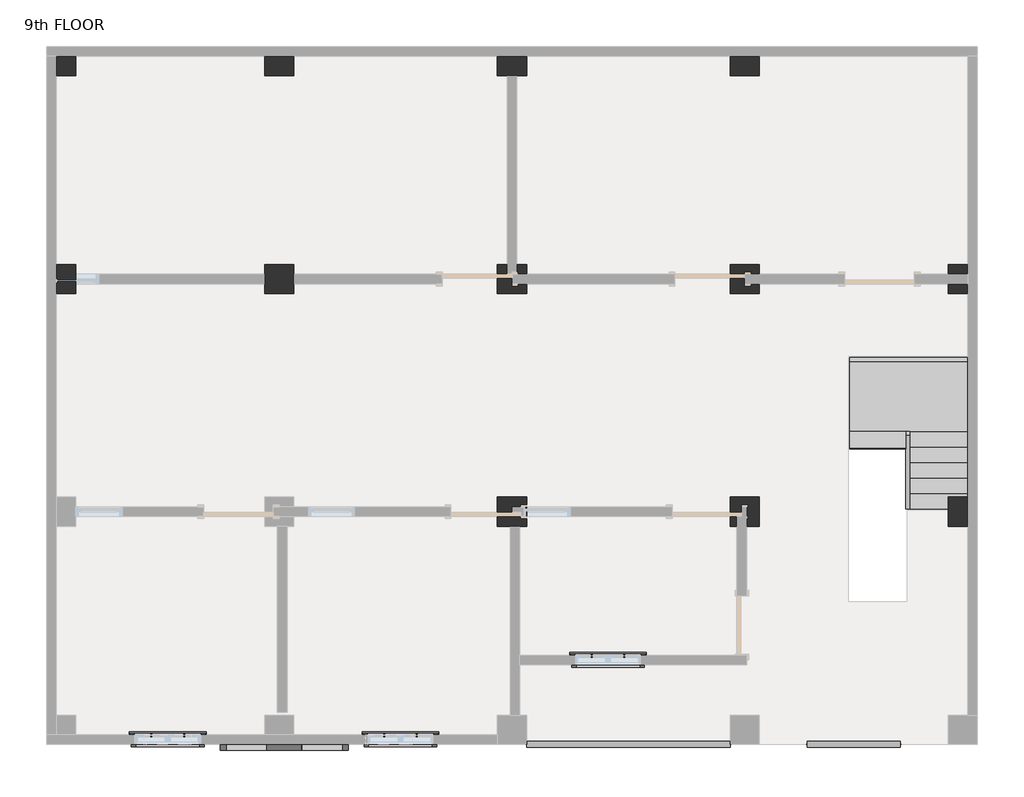
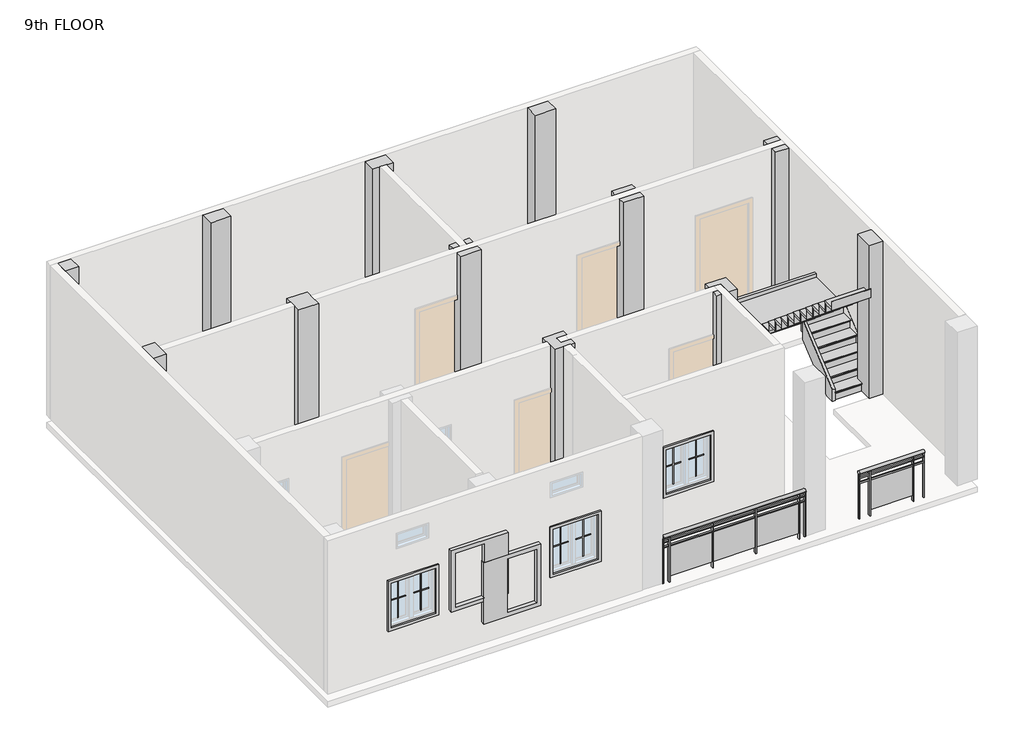
# One storey, part 2 of 2: 12 columns, 12 proxies, 4 members, 2 railings, 1 damper, 1 stair flight.
"""IFC4 building model written with IfcOpenShell, lengths in millimetres."""

from ifc_helpers import new_model, si_unit, point, frame, origin, place, context, project, spatial, polyline, ellipse_curve, trimmed, outline, extrude, faceted_brep, transform, mapped, element, save
from ifc_brep_helpers import plane_surface, extruded_surface, advanced_brep
from components import muntin_pattern_2x2_muntin_pattern_2x2_b3fe6957, muntin_pattern_2x2_muntin_pattern_2x2_3e0ecaf2, trim_window_exterior_flat_with_sill_41619996, trim_window_interior_flat_picture_frame_51c85655, duct_accessories_4_duct_accessories_1_42753040, stair_flight_cacad448

model = new_model("IFC4")

# Units and contexts
model_context = context("Model", 3, world=origin())
ifc_project = project(units=[si_unit("LENGTHUNIT", "METRE", prefix="MILLI")], contexts=[model_context])

# Site, building, storey
site = spatial("IfcSite", under=ifc_project)
building = spatial("IfcBuilding", under=site)
storey = spatial("IfcBuildingStorey", under=building, Name="9th FLOOR", Elevation=27279.6)

# Proxies
placement = place(None, origin())
muntin_pattern_2x2_muntin_pattern_2x2_shape = muntin_pattern_2x2_muntin_pattern_2x2_b3fe6957(model_context)
element("IfcBuildingElementProxy", 1, Name="Muntin Pattern_2x2 : Muntin Pattern_2x2", ObjectType="Muntin Pattern_2x2 : Muntin Pattern_2x2", at=placement, inside=storey, context=model_context, shape_type="MappedRepresentation", body=[
    mapped(muntin_pattern_2x2_muntin_pattern_2x2_shape, transform((-14441.409625, -253.8184478, 28263.85), x_axis=(1.0, 0.0, 0.0), y_axis=(0.0, 1.0, 0.0), z_axis=(0.0, 0.0, 1.0))),
])
element("IfcBuildingElementProxy", 2, Name="Muntin Pattern_2x2 : Muntin Pattern_2x2", ObjectType="Muntin Pattern_2x2 : Muntin Pattern_2x2", at=placement, inside=storey, context=model_context, shape_type="MappedRepresentation", body=[
    mapped(muntin_pattern_2x2_muntin_pattern_2x2_shape, transform((-11393.409625, -253.8184478, 28263.85), x_axis=(1.0, 0.0, 0.0), y_axis=(0.0, 1.0, 0.0), z_axis=(0.0, 0.0, 1.0))),
])
element("IfcBuildingElementProxy", 3, Name="Muntin Pattern_2x2 : Muntin Pattern_2x2", ObjectType="Muntin Pattern_2x2 : Muntin Pattern_2x2", at=placement, inside=storey, context=model_context, shape_type="MappedRepresentation", body=[
    mapped(muntin_pattern_2x2_muntin_pattern_2x2_shape, transform((-8675.609625, 787.5815522, 28263.85), x_axis=(1.0, 0.0, 0.0), y_axis=(0.0, 1.0, 0.0), z_axis=(0.0, 0.0, 1.0))),
])
muntin_pattern_2x2_muntin_pattern_2x2_2_shape = muntin_pattern_2x2_muntin_pattern_2x2_3e0ecaf2(model_context)
element("IfcBuildingElementProxy", 4, Name="Muntin Pattern_2x2 : Muntin Pattern_2x2", ObjectType="Muntin Pattern_2x2 : Muntin Pattern_2x2", at=placement, inside=storey, context=model_context, shape_type="MappedRepresentation", body=[
    mapped(muntin_pattern_2x2_muntin_pattern_2x2_2_shape, transform((-14012.784625, -253.8184478, 28263.85), x_axis=(-1.0, 0.0, 0.0), y_axis=(0.0, -1.0, 0.0), z_axis=(0.0, 0.0, 1.0))),
])
element("IfcBuildingElementProxy", 5, Name="Muntin Pattern_2x2 : Muntin Pattern_2x2", ObjectType="Muntin Pattern_2x2 : Muntin Pattern_2x2", at=placement, inside=storey, context=model_context, shape_type="MappedRepresentation", body=[
    mapped(muntin_pattern_2x2_muntin_pattern_2x2_2_shape, transform((-10964.784625, -253.8184478, 28263.85), x_axis=(-1.0, 0.0, 0.0), y_axis=(0.0, -1.0, 0.0), z_axis=(0.0, 0.0, 1.0))),
])
element("IfcBuildingElementProxy", 6, Name="Muntin Pattern_2x2 : Muntin Pattern_2x2", ObjectType="Muntin Pattern_2x2 : Muntin Pattern_2x2", at=placement, inside=storey, context=model_context, shape_type="MappedRepresentation", body=[
    mapped(muntin_pattern_2x2_muntin_pattern_2x2_2_shape, transform((-8246.984625, 787.5815522, 28263.85), x_axis=(-1.0, 0.0, 0.0), y_axis=(0.0, -1.0, 0.0), z_axis=(0.0, 0.0, 1.0))),
])
trim_window_exterior_flat_with_sill_shape = trim_window_exterior_flat_with_sill_41619996(model_context)
element("IfcBuildingElementProxy", 7, Name="Trim-Window-Exterior-Flat : with Sill", ObjectType="Trim-Window-Exterior-Flat : with Sill", at=placement, inside=storey, context=model_context, shape_type="MappedRepresentation", body=[
    mapped(trim_window_exterior_flat_with_sill_shape, transform((-14227.097125, -244.2934478, 29108.4), x_axis=(-1.0, 0.0, 0.0), y_axis=(0.0, 0.0, 1.0), z_axis=(0.0, 1.0, 0.0))),
])
element("IfcBuildingElementProxy", 8, Name="Trim-Window-Exterior-Flat : with Sill", ObjectType="Trim-Window-Exterior-Flat : with Sill", at=placement, inside=storey, context=model_context, shape_type="MappedRepresentation", body=[
    mapped(trim_window_exterior_flat_with_sill_shape, transform((-11179.097125, -244.2934478, 29108.4), x_axis=(-1.0, 0.0, 0.0), y_axis=(0.0, 0.0, 1.0), z_axis=(0.0, 1.0, 0.0))),
])
element("IfcBuildingElementProxy", 9, Name="Trim-Window-Exterior-Flat : with Sill", ObjectType="Trim-Window-Exterior-Flat : with Sill", at=placement, inside=storey, context=model_context, shape_type="MappedRepresentation", body=[
    mapped(trim_window_exterior_flat_with_sill_shape, transform((-8461.297125, 797.1065522, 29108.4), x_axis=(-1.0, 0.0, 0.0), y_axis=(0.0, 0.0, 1.0), z_axis=(0.0, 1.0, 0.0))),
])
trim_window_interior_flat_picture_frame_shape = trim_window_interior_flat_picture_frame_51c85655(model_context)
element("IfcBuildingElementProxy", 10, Name="Trim-Window-Interior-Flat : Picture Frame", ObjectType="Trim-Window-Interior-Flat : Picture Frame", at=placement, inside=storey, context=model_context, shape_type="MappedRepresentation", body=[
    mapped(trim_window_interior_flat_picture_frame_shape, transform((-14227.097125, -371.2934478, 29108.4), x_axis=(1.0, 0.0, 0.0), y_axis=(0.0, 0.0, 1.0), z_axis=(0.0, -1.0, 0.0))),
])
element("IfcBuildingElementProxy", 11, Name="Trim-Window-Interior-Flat : Picture Frame", ObjectType="Trim-Window-Interior-Flat : Picture Frame", at=placement, inside=storey, context=model_context, shape_type="MappedRepresentation", body=[
    mapped(trim_window_interior_flat_picture_frame_shape, transform((-11179.097125, -371.2934478, 29108.4), x_axis=(1.0, 0.0, 0.0), y_axis=(0.0, 0.0, 1.0), z_axis=(0.0, -1.0, 0.0))),
])
element("IfcBuildingElementProxy", 12, Name="Trim-Window-Interior-Flat : Picture Frame", ObjectType="Trim-Window-Interior-Flat : Picture Frame", at=placement, inside=storey, context=model_context, shape_type="MappedRepresentation", body=[
    mapped(trim_window_interior_flat_picture_frame_shape, transform((-8461.297125, 670.1065522, 29108.4), x_axis=(1.0, 0.0, 0.0), y_axis=(0.0, 0.0, 1.0), z_axis=(0.0, -1.0, 0.0))),
])

# Columns
element("IfcColumn", 13, ObjectType="column family : column family", at=placement, inside=storey, context=model_context, shape_type="SweptSolid", body=[
    extrude(outline(polyline([(-15433.597125, 8645.7065522), (-15433.597125, 8391.7065522), (-15687.597125, 8391.7065522), (-15687.597125, 8645.7065522), (-15433.597125, 8645.7065522)])), frame((0.0, 0.0, 27284.6), z_axis=(0.0, 0.0, 1.0), x_axis=(1.0, 0.0, 0.0)), (0.0, 0.0, 1.0), 3038.0),
])
element("IfcColumn", 14, ObjectType="column family : column family", at=placement, inside=storey, context=model_context, shape_type="SweptSolid", body=[
    extrude(outline(polyline([(-12576.097125, 5915.2065522), (-12576.097125, 5534.2065522), (-12957.097125, 5534.2065522), (-12957.097125, 5915.2065522), (-12576.097125, 5915.2065522)])), frame((0.0, 0.0, 27284.6), z_axis=(0.0, 0.0, 1.0), x_axis=(1.0, 0.0, 0.0)), (0.0, 0.0, 1.0), 3038.0),
])
element("IfcColumn", 15, ObjectType="column family : column family", at=placement, inside=storey, context=model_context, shape_type="Brep", body=[
    faceted_brep([(-9655.097125, 5915.2065522, 27284.6), (-9528.097125, 5915.2065522, 27284.6), (-9528.097125, 5788.2065522, 27284.6), (-9655.097125, 5788.2065522, 27284.6), (-9528.097125, 5915.2065522, 30322.6), (-9655.097125, 5915.2065522, 30322.6), (-9655.097125, 5788.2065522, 30322.6), (-9528.097125, 5788.2065522, 30322.6)], [[[0, 1, 2, 3]], [[4, 5, 6, 7]], [[0, 3, 6, 5]], [[4, 1, 0, 5]], [[3, 2, 7, 6]], [[1, 4, 7, 2]]]),
    faceted_brep([(-9528.097125, 5534.2065522, 30322.6), (-9528.097125, 5534.2065522, 27284.6), (-9528.097125, 5661.2065522, 27284.6), (-9528.097125, 5661.2065522, 30322.6), (-9909.097125, 5534.2065522, 27284.6), (-9909.097125, 5534.2065522, 30322.6), (-9909.097125, 5915.2065522, 27284.6), (-9909.097125, 5661.2065522, 30322.6), (-9909.097125, 5661.2065522, 29413.2), (-9909.097125, 5788.2065522, 29413.2), (-9909.097125, 5788.2065522, 30322.6), (-9909.097125, 5915.2065522, 30322.6), (-9782.097125, 5915.2065522, 30322.6), (-9782.097125, 5915.2065522, 27284.6), (-9782.097125, 5788.2065522, 27284.6), (-9782.097125, 5788.2065522, 30322.6), (-9782.097125, 5788.2065522, 29413.2), (-9718.597125, 5788.2065522, 27284.6), (-9718.597125, 5788.2065522, 29413.2), (-9718.597125, 5661.2065522, 27284.6), (-9718.597125, 5661.2065522, 29413.2)], [[[0, 1, 2, 3]], [[4, 1, 0, 5]], [[6, 4, 5, 7, 8, 9, 10, 11]], [[6, 11, 12, 13]], [[14, 13, 12, 15, 16]], [[17, 14, 16, 18]], [[19, 20, 8, 7, 3, 2]], [[1, 4, 6, 13, 14, 17, 19, 2]], [[5, 0, 3, 7]], [[12, 11, 10, 15]], [[9, 16, 15, 10]], [[18, 20, 19, 17]], [[20, 18, 16, 9, 8]]]),
])
element("IfcColumn", 16, ObjectType="column family : column family", at=placement, inside=storey, context=model_context, shape_type="Brep", body=[
    faceted_brep([(-6480.097125, 5534.2065522, 27284.6), (-6861.097125, 5534.2065522, 27284.6), (-6861.097125, 5915.2065522, 27284.6), (-6480.097125, 5915.2065522, 27284.6), (-6480.097125, 5788.2065522, 27284.6), (-6670.597125, 5788.2065522, 27284.6), (-6670.597125, 5661.2065522, 27284.6), (-6480.097125, 5661.2065522, 27284.6), (-6480.097125, 5534.2065522, 30322.6), (-6480.097125, 5661.2065522, 30322.6), (-6861.097125, 5534.2065522, 30322.6), (-6861.097125, 5661.2065522, 30322.6), (-6861.097125, 5661.2065522, 29413.2), (-6861.097125, 5788.2065522, 29413.2), (-6861.097125, 5788.2065522, 30322.6), (-6861.097125, 5915.2065522, 30322.6), (-6480.097125, 5915.2065522, 30322.6), (-6670.597125, 5661.2065522, 29413.2), (-6670.597125, 5788.2065522, 29413.2), (-6480.097125, 5788.2065522, 30322.6)], [[[0, 1, 2, 3, 4, 5, 6, 7]], [[8, 0, 7, 9]], [[1, 0, 8, 10]], [[2, 1, 10, 11, 12, 13, 14, 15]], [[3, 2, 15, 16]], [[10, 8, 9, 11]], [[6, 17, 12, 11, 9, 7]], [[13, 18, 5, 4, 19, 14]], [[3, 16, 19, 4]], [[16, 15, 14, 19]], [[18, 17, 6, 5]], [[17, 18, 13, 12]]]),
])
element("IfcColumn", 17, ObjectType="column family : column family", at=placement, inside=storey, context=model_context, shape_type="Brep", body=[
    faceted_brep([(-6480.097125, 2867.2065522, 27284.6), (-6480.097125, 2486.2065522, 27284.6), (-6645.197125, 2486.2065522, 27284.6), (-6645.197125, 2740.2065522, 27284.6), (-6708.697125, 2740.2065522, 27284.6), (-6708.697125, 2613.2065522, 27284.6), (-6772.197125, 2613.2065522, 27284.6), (-6772.197125, 2486.2065522, 27284.6), (-6861.097125, 2486.2065522, 27284.6), (-6861.097125, 2867.2065522, 27284.6), (-6480.097125, 2867.2065522, 30322.6), (-6480.097125, 2486.2065522, 30322.6), (-6861.097125, 2486.2065522, 30322.6), (-6772.197125, 2486.2065522, 30322.6), (-6861.097125, 2613.2065522, 30322.6), (-6861.097125, 2613.2065522, 29413.2), (-6861.097125, 2740.2065522, 29413.2), (-6861.097125, 2740.2065522, 30322.6), (-6861.097125, 2867.2065522, 30322.6), (-6772.197125, 2740.2065522, 30322.6), (-6645.197125, 2740.2065522, 30322.6), (-6645.197125, 2486.2065522, 30322.6), (-6772.197125, 2613.2065522, 30322.6), (-6772.197125, 2613.2065522, 29413.2), (-6772.197125, 2740.2065522, 29413.2), (-6708.697125, 2613.2065522, 29413.2), (-6708.697125, 2740.2065522, 29413.2)], [[[0, 1, 2, 3, 4, 5, 6, 7, 8, 9]], [[1, 0, 10, 11]], [[12, 8, 7, 13]], [[9, 8, 12, 14, 15, 16, 17, 18]], [[0, 9, 18, 10]], [[11, 10, 18, 17, 19, 20, 21]], [[15, 14, 22, 23]], [[17, 16, 24, 19]], [[20, 3, 2, 21]], [[6, 23, 22, 13, 7]], [[14, 12, 13, 22]], [[1, 11, 21, 2]], [[15, 23, 24, 16]], [[25, 23, 6, 5]], [[23, 25, 26, 24]], [[26, 25, 5, 4]], [[24, 26, 4, 3, 20, 19]]]),
])
element("IfcColumn", 18, ObjectType="column family : column family", at=placement, inside=storey, context=model_context, shape_type="Brep", body=[
    faceted_brep([(-9528.097125, 2486.2065522, 27284.6), (-9909.097125, 2486.2065522, 27284.6), (-9909.097125, 2867.2065522, 27284.6), (-9528.097125, 2867.2065522, 27284.6), (-9528.097125, 2740.2065522, 27284.6), (-9566.197125, 2740.2065522, 27284.6), (-9718.597125, 2740.2065522, 27284.6), (-9718.597125, 2613.2065522, 27284.6), (-9566.197125, 2613.2065522, 27284.6), (-9528.097125, 2613.2065522, 27284.6), (-9528.097125, 2486.2065522, 30322.6), (-9528.097125, 2613.2065522, 27584.4), (-9528.097125, 2740.2065522, 27584.4), (-9528.097125, 2867.2065522, 30322.6), (-9528.097125, 2740.2065522, 30322.6), (-9528.097125, 2740.2065522, 29413.2), (-9528.097125, 2613.2065522, 29413.2), (-9528.097125, 2613.2065522, 30322.6), (-9909.097125, 2486.2065522, 30322.6), (-9909.097125, 2867.2065522, 30322.6), (-9566.197125, 2613.2065522, 30322.6), (-9718.597125, 2613.2065522, 30322.6), (-9718.597125, 2740.2065522, 30322.6), (-9566.197125, 2740.2065522, 30322.6), (-9566.197125, 2613.2065522, 29413.2), (-9566.197125, 2613.2065522, 27584.4), (-9566.197125, 2740.2065522, 27584.4), (-9566.197125, 2740.2065522, 29413.2)], [[[0, 1, 2, 3, 4, 5, 6, 7, 8, 9]], [[10, 0, 9, 11, 12, 4, 3, 13, 14, 15, 16, 17]], [[1, 0, 10, 18]], [[2, 1, 18, 19]], [[3, 2, 19, 13]], [[18, 10, 17, 20, 21, 22, 23, 14, 13, 19]], [[11, 9, 8, 7, 21, 20, 17, 16, 24, 25]], [[4, 12, 26, 27, 15, 14, 23, 22, 6, 5]], [[21, 7, 6, 22]], [[25, 24, 27, 26]], [[25, 26, 12, 11]], [[27, 24, 16, 15]]]),
])
element("IfcColumn", 19, ObjectType="column family : column family", at=placement, inside=storey, context=model_context, shape_type="SweptSolid", body=[
    extrude(outline(polyline([(-12576.097125, 8391.7065522), (-12957.097125, 8391.7065522), (-12957.097125, 8645.7065522), (-12576.097125, 8645.7065522), (-12576.097125, 8391.7065522)])), frame((0.0, 0.0, 27284.6), z_axis=(0.0, 0.0, 1.0), x_axis=(1.0, 0.0, 0.0)), (0.0, 0.0, 1.0), 3038.0),
])
element("IfcColumn", 20, ObjectType="column family : column family", at=placement, inside=storey, context=model_context, shape_type="SweptSolid", body=[
    extrude(outline(polyline([(-9528.097125, 8391.7065522), (-9909.097125, 8391.7065522), (-9909.097125, 8645.7065522), (-9528.097125, 8645.7065522), (-9528.097125, 8391.7065522)])), frame((0.0, 0.0, 27284.6), z_axis=(0.0, 0.0, 1.0), x_axis=(1.0, 0.0, 0.0)), (0.0, 0.0, 1.0), 3038.0),
])
element("IfcColumn", 21, ObjectType="column family : column family", at=placement, inside=storey, context=model_context, shape_type="SweptSolid", body=[
    extrude(outline(polyline([(-6480.097125, 8391.7065522), (-6861.097125, 8391.7065522), (-6861.097125, 8645.7065522), (-6480.097125, 8645.7065522), (-6480.097125, 8391.7065522)])), frame((0.0, 0.0, 27284.6), z_axis=(0.0, 0.0, 1.0), x_axis=(1.0, 0.0, 0.0)), (0.0, 0.0, 1.0), 3038.0),
])
element("IfcColumn", 22, ObjectType="column family : column family", at=placement, inside=storey, context=model_context, shape_type="SweptSolid", body=[
    extrude(outline(polyline([(-4003.597125, 5915.2065522), (-3749.597125, 5915.2065522), (-3749.597125, 5788.2065522), (-4003.597125, 5788.2065522), (-4003.597125, 5915.2065522)])), frame((0.0, 0.0, 27284.6), z_axis=(0.0, 0.0, 1.0), x_axis=(1.0, 0.0, 0.0)), (0.0, 0.0, 1.0), 3038.0),
    extrude(outline(polyline([(-3749.597125, 5534.2065522), (-4003.597125, 5534.2065522), (-4003.597125, 5661.2065522), (-3749.597125, 5661.2065522), (-3749.597125, 5534.2065522)])), frame((0.0, 0.0, 27284.6), z_axis=(0.0, 0.0, 1.0), x_axis=(1.0, 0.0, 0.0)), (0.0, 0.0, 1.0), 3038.0),
])
element("IfcColumn", 23, ObjectType="column family : column family", at=placement, inside=storey, context=model_context, shape_type="SweptSolid", body=[
    extrude(outline(polyline([(-4003.597125, 2486.2065522), (-4003.597125, 2867.2065522), (-3749.597125, 2867.2065522), (-3749.597125, 2486.2065522), (-4003.597125, 2486.2065522)])), frame((0.0, 0.0, 27284.6), z_axis=(0.0, 0.0, 1.0), x_axis=(1.0, 0.0, 0.0)), (0.0, 0.0, 1.0), 3038.0),
])
element("IfcColumn", 24, ObjectType="column family : column family", at=placement, inside=storey, context=model_context, shape_type="SweptSolid", body=[
    extrude(outline(polyline([(-15433.597125, 5915.2065522), (-15433.597125, 5534.2065522), (-15687.597125, 5534.2065522), (-15687.597125, 5915.2065522), (-15433.597125, 5915.2065522)])), frame((0.0, 0.0, 27284.6), z_axis=(0.0, 0.0, 1.0), x_axis=(1.0, 0.0, 0.0)), (0.0, 0.0, 1.0), 3038.0),
])

# Damper
duct_accessories_4_duct_accessories_1_shape = duct_accessories_4_duct_accessories_1_42753040(model_context)
element("IfcDamper", 25, ObjectType="Duct Accessories 4 : Duct Accessories 1", at=placement, inside=storey, context=model_context, shape_type="MappedRepresentation", body=[
    mapped(duct_accessories_4_duct_accessories_1_shape, transform((0.0, 0.0, 0.0), x_axis=(1.0, 0.0, 0.0), y_axis=(0.0, 1.0, 0.0), z_axis=(0.0, 0.0, 1.0))),
])

# Members
element("IfcMember", 26, ObjectType="Stringer - 2\" Width", at=placement, inside=storey, context=model_context, shape_type="SweptSolid", body=[
    extrude(outline(polyline([(2714.6319226, 27279.6), (2714.6319226, 27516.4438745), (3679.8319226, 28320.7772078), (3679.8319226, 27924.0165243), (2906.5320935, 27279.6), (2714.6319226, 27279.6)])), frame((-4563.0136682, 0.0, 0.0), z_axis=(1.0, 0.0, 0.0), x_axis=(0.0, 1.0, 0.0)), (0.0, 0.0, 1.0), 50.8),
])
element("IfcMember", 27, ObjectType="Stringer - 2\" Width", at=placement, inside=storey, context=model_context, shape_type="SweptSolid", body=[
    extrude(outline(polyline([(-4512.2136682, 3730.6319226), (-4512.2136682, 3679.8319226), (-4563.0136682, 3679.8319226), (-4563.0136682, 3730.6319226), (-4512.2136682, 3730.6319226)])), frame((0.0, 0.0, 28067.0), z_axis=(0.0, 0.0, 1.0), x_axis=(1.0, 0.0, 0.0)), (0.0, 0.0, 1.0), 304.8),
])
element("IfcMember", 28, ObjectType="Stringer - 2\" Width", at=placement, inside=storey, context=model_context, shape_type="SweptSolid", body=[
    extrude(outline(polyline([(2714.6319226, 27279.6), (2714.6319226, 27516.4438745), (3741.0592732, 28371.8), (4217.1720935, 28371.8), (2906.5320935, 27279.6), (2714.6319226, 27279.6)])), frame((-3749.597125, 0.0, 0.0), z_axis=(1.0, 0.0, 0.0), x_axis=(0.0, 1.0, 0.0)), (0.0, 0.0, 1.0), 50.8),
])
element("IfcMember", 29, ObjectType="Stringer - 2\" Width", at=placement, inside=storey, context=model_context, shape_type="SweptSolid", body=[
    extrude(outline(polyline([(-3698.797125, 4695.8319226), (-3698.797125, 4645.0319226), (-5295.0246464, 4645.0319226), (-5295.0246464, 4695.8319226), (-3698.797125, 4695.8319226)])), frame((0.0, 0.0, 28067.0), z_axis=(0.0, 0.0, 1.0), x_axis=(1.0, 0.0, 0.0)), (0.0, 0.0, 1.0), 304.8),
])

# Railings
element("IfcRailing", 30, ObjectType="Glass Panel - Bottom Fill", at=placement, inside=storey, context=model_context, shape_type="SolidModel", body=[
    advanced_brep(
    [(-9528.097125, -333.1934478, 28194.0), (-9528.097125, -409.3934478, 28194.0), (-6861.097125, -333.1934478, 28194.0), (-6861.097125, -409.3934478, 28194.0)],
    [
        (0, 1, ellipse_curve(frame((-9528.097125, -371.2934478, 28194.0), z_axis=(-1.0, 0.0, 0.0), x_axis=(0.0, -1.0, 0.0)), 38.1, 28.575)),
        (1, 0, ellipse_curve(frame((-9528.097125, -371.2934478, 28194.0), z_axis=(-1.0, 0.0, 0.0), x_axis=(0.0, -1.0, 0.0)), 38.1, 28.575)),
        (2, 3, ellipse_curve(frame((-6861.097125, -371.2934478, 28194.0), z_axis=(1.0, 0.0, 0.0), x_axis=(0.0, -1.0, 0.0)), 38.1, 28.575)),
        (3, 2, ellipse_curve(frame((-6861.097125, -371.2934478, 28194.0), z_axis=(1.0, 0.0, 0.0), x_axis=(0.0, -1.0, 0.0)), 38.1, 28.575)),
        (0, 2),
        (3, 1),
    ],
    [
        plane_surface(frame((-9528.097125, -371.2934478, 28194.0), z_axis=(-1.0, 0.0, 0.0), x_axis=(0.0, 1.0, 0.0))),
        plane_surface(frame((-6861.097125, -371.2934478, 28194.0), z_axis=(1.0, 0.0, 0.0), x_axis=(0.0, 1.0, 0.0))),
        extruded_surface(trimmed(ellipse_curve(frame((-6861.097125, -371.2934478, 28194.0), z_axis=(-1.0, 0.0, 0.0), x_axis=(0.0, -1.0, 0.0)), 38.1, 28.575), [point((-6861.097125, -333.1934478, 28194.0))], [point((-6861.097125, -409.3934478, 28194.0))], True, "CARTESIAN"), (-2667.0, 0.0, 0.0), 2667.0),
        extruded_surface(trimmed(ellipse_curve(frame((-6861.097125, -371.2934478, 28194.0), z_axis=(-1.0, 0.0, 0.0), x_axis=(0.0, -1.0, 0.0)), 38.1, 28.575), [point((-6861.097125, -409.3934478, 28194.0))], [point((-6861.097125, -333.1934478, 28194.0))], True, "CARTESIAN"), (-2667.0, 0.0, 0.0), 2667.0),
    ],
    [
        (0, [[1, 2]]),
        (1, [[3, 4]]),
        (2, [[-1, 5, -4, 6]]),
        (3, [[-2, -6, -3, -5]]),
    ],
),
    extrude(outline(polyline([(-9528.097125, -383.9934478), (-9528.097125, -358.5934478), (-6861.097125, -358.5934478), (-6861.097125, -383.9934478), (-9528.097125, -383.9934478)])), frame((0.0, 0.0, 28079.7), z_axis=(0.0, 0.0, 1.0), x_axis=(1.0, 0.0, 0.0)), (0.0, 0.0, 1.0), 25.4),
    extrude(outline(polyline([(-9528.097125, -383.9934478), (-9528.097125, -358.5934478), (-6861.097125, -358.5934478), (-6861.097125, -383.9934478), (-9528.097125, -383.9934478)])), frame((0.0, 0.0, 27978.1), z_axis=(0.0, 0.0, 1.0), x_axis=(1.0, 0.0, 0.0)), (0.0, 0.0, 1.0), 25.4),
    extrude(outline(polyline([(-6981.747125, -396.6934478), (-6981.747125, -345.8934478), (-6969.047125, -345.8934478), (-6969.047125, -396.6934478), (-6981.747125, -396.6934478)])), frame((0.0, 0.0, 27279.6), z_axis=(0.0, 0.0, 1.0), x_axis=(1.0, 0.0, 0.0)), (0.0, 0.0, 1.0), 885.6788223),
    extrude(outline(polyline([(-7788.197125, -364.7582908), (-6975.397125, -364.7582908), (-6975.397125, -371.1082908), (-7788.197125, -371.1082908), (-7788.197125, -364.7582908)])), frame((0.0, 0.0, 27381.2), z_axis=(0.0, 0.0, 1.0), x_axis=(1.0, 0.0, 0.0)), (0.0, 0.0, 1.0), 596.9),
    extrude(outline(polyline([(-7794.547125, -396.6934478), (-7794.547125, -345.8934478), (-7781.847125, -345.8934478), (-7781.847125, -396.6934478), (-7794.547125, -396.6934478)])), frame((0.0, 0.0, 27279.6), z_axis=(0.0, 0.0, 1.0), x_axis=(1.0, 0.0, 0.0)), (0.0, 0.0, 1.0), 885.6788223),
    extrude(outline(polyline([(-8600.997125, -364.7582908), (-7788.197125, -364.7582908), (-7788.197125, -371.1082908), (-8600.997125, -371.1082908), (-8600.997125, -364.7582908)])), frame((0.0, 0.0, 27381.2), z_axis=(0.0, 0.0, 1.0), x_axis=(1.0, 0.0, 0.0)), (0.0, 0.0, 1.0), 596.9),
    extrude(outline(polyline([(-8607.347125, -396.6934478), (-8607.347125, -345.8934478), (-8594.647125, -345.8934478), (-8594.647125, -396.6934478), (-8607.347125, -396.6934478)])), frame((0.0, 0.0, 27279.6), z_axis=(0.0, 0.0, 1.0), x_axis=(1.0, 0.0, 0.0)), (0.0, 0.0, 1.0), 885.6788223),
    extrude(outline(polyline([(-9413.797125, -364.7582908), (-8600.997125, -364.7582908), (-8600.997125, -371.1082908), (-9413.797125, -371.1082908), (-9413.797125, -364.7582908)])), frame((0.0, 0.0, 27381.2), z_axis=(0.0, 0.0, 1.0), x_axis=(1.0, 0.0, 0.0)), (0.0, 0.0, 1.0), 596.9),
    extrude(outline(polyline([(-9420.147125, -396.6934478), (-9420.147125, -345.8934478), (-9407.447125, -345.8934478), (-9407.447125, -396.6934478), (-9420.147125, -396.6934478)])), frame((0.0, 0.0, 27279.6), z_axis=(0.0, 0.0, 1.0), x_axis=(1.0, 0.0, 0.0)), (0.0, 0.0, 1.0), 885.6788223),
    extrude(outline(polyline([(-6873.797125, -380.8184478), (-6873.797125, -361.7684478), (-6854.747125, -361.7684478), (-6854.747125, -380.8184478), (-6873.797125, -380.8184478)])), frame((0.0, 0.0, 27279.6), z_axis=(0.0, 0.0, 1.0), x_axis=(1.0, 0.0, 0.0)), (0.0, 0.0, 1.0), 885.6788223),
    extrude(outline(polyline([(-9534.447125, -380.8184478), (-9534.447125, -361.7684478), (-9515.397125, -361.7684478), (-9515.397125, -380.8184478), (-9534.447125, -380.8184478)])), frame((0.0, 0.0, 27279.6), z_axis=(0.0, 0.0, 1.0), x_axis=(1.0, 0.0, 0.0)), (0.0, 0.0, 1.0), 885.6788223),
])
element("IfcRailing", 31, ObjectType="Glass Panel - Bottom Fill", at=placement, inside=storey, context=model_context, shape_type="SolidModel", body=[
    advanced_brep(
    [(-5851.447125, -333.1934478, 28194.0), (-5851.447125, -409.3934478, 28194.0), (-4632.247125, -333.1934478, 28194.0), (-4632.247125, -409.3934478, 28194.0)],
    [
        (0, 1, ellipse_curve(frame((-5851.447125, -371.2934478, 28194.0), z_axis=(-1.0, 0.0, 0.0), x_axis=(0.0, -1.0, 0.0)), 38.1, 28.575)),
        (1, 0, ellipse_curve(frame((-5851.447125, -371.2934478, 28194.0), z_axis=(-1.0, 0.0, 0.0), x_axis=(0.0, -1.0, 0.0)), 38.1, 28.575)),
        (2, 3, ellipse_curve(frame((-4632.247125, -371.2934478, 28194.0), z_axis=(1.0, 0.0, 0.0), x_axis=(0.0, -1.0, 0.0)), 38.1, 28.575)),
        (3, 2, ellipse_curve(frame((-4632.247125, -371.2934478, 28194.0), z_axis=(1.0, 0.0, 0.0), x_axis=(0.0, -1.0, 0.0)), 38.1, 28.575)),
        (0, 2),
        (3, 1),
    ],
    [
        plane_surface(frame((-5851.447125, -371.2934478, 28194.0), z_axis=(-1.0, 0.0, 0.0), x_axis=(0.0, 1.0, 0.0))),
        plane_surface(frame((-4632.247125, -371.2934478, 28194.0), z_axis=(1.0, 0.0, 0.0), x_axis=(0.0, 1.0, 0.0))),
        extruded_surface(trimmed(ellipse_curve(frame((-4632.247125, -371.2934478, 28194.0), z_axis=(-1.0, 0.0, 0.0), x_axis=(0.0, -1.0, 0.0)), 38.1, 28.575), [point((-4632.247125, -333.1934478, 28194.0))], [point((-4632.247125, -409.3934478, 28194.0))], True, "CARTESIAN"), (-1219.1999999999998, 0.0, 0.0), 1219.1999999999998),
        extruded_surface(trimmed(ellipse_curve(frame((-4632.247125, -371.2934478, 28194.0), z_axis=(-1.0, 0.0, 0.0), x_axis=(0.0, -1.0, 0.0)), 38.1, 28.575), [point((-4632.247125, -409.3934478, 28194.0))], [point((-4632.247125, -333.1934478, 28194.0))], True, "CARTESIAN"), (-1219.1999999999998, 0.0, 0.0), 1219.1999999999998),
    ],
    [
        (0, [[1, 2]]),
        (1, [[3, 4]]),
        (2, [[-1, 5, -4, 6]]),
        (3, [[-2, -6, -3, -5]]),
    ],
),
    extrude(outline(polyline([(-5851.447125, -383.9934478), (-5851.447125, -358.5934478), (-4632.247125, -358.5934478), (-4632.247125, -383.9934478), (-5851.447125, -383.9934478)])), frame((0.0, 0.0, 28079.7), z_axis=(0.0, 0.0, 1.0), x_axis=(1.0, 0.0, 0.0)), (0.0, 0.0, 1.0), 25.4),
    extrude(outline(polyline([(-5851.447125, -383.9934478), (-5851.447125, -358.5934478), (-4632.247125, -358.5934478), (-4632.247125, -383.9934478), (-5851.447125, -383.9934478)])), frame((0.0, 0.0, 27978.1), z_axis=(0.0, 0.0, 1.0), x_axis=(1.0, 0.0, 0.0)), (0.0, 0.0, 1.0), 25.4),
    extrude(outline(polyline([(-4841.797125, -396.6934478), (-4841.797125, -345.8934478), (-4829.097125, -345.8934478), (-4829.097125, -396.6934478), (-4841.797125, -396.6934478)])), frame((0.0, 0.0, 27279.6), z_axis=(0.0, 0.0, 1.0), x_axis=(1.0, 0.0, 0.0)), (0.0, 0.0, 1.0), 885.6788223),
    extrude(outline(polyline([(-5648.247125, -364.7582908), (-4835.447125, -364.7582908), (-4835.447125, -371.1082908), (-5648.247125, -371.1082908), (-5648.247125, -364.7582908)])), frame((0.0, 0.0, 27381.2), z_axis=(0.0, 0.0, 1.0), x_axis=(1.0, 0.0, 0.0)), (0.0, 0.0, 1.0), 596.9),
    extrude(outline(polyline([(-5654.597125, -396.6934478), (-5654.597125, -345.8934478), (-5641.897125, -345.8934478), (-5641.897125, -396.6934478), (-5654.597125, -396.6934478)])), frame((0.0, 0.0, 27279.6), z_axis=(0.0, 0.0, 1.0), x_axis=(1.0, 0.0, 0.0)), (0.0, 0.0, 1.0), 885.6788223),
    extrude(outline(polyline([(-4644.947125, -380.8184478), (-4644.947125, -361.7684478), (-4625.897125, -361.7684478), (-4625.897125, -380.8184478), (-4644.947125, -380.8184478)])), frame((0.0, 0.0, 27279.6), z_axis=(0.0, 0.0, 1.0), x_axis=(1.0, 0.0, 0.0)), (0.0, 0.0, 1.0), 885.6788223),
    extrude(outline(polyline([(-5857.797125, -380.8184478), (-5857.797125, -361.7684478), (-5838.747125, -361.7684478), (-5838.747125, -380.8184478), (-5857.797125, -380.8184478)])), frame((0.0, 0.0, 27279.6), z_axis=(0.0, 0.0, 1.0), x_axis=(1.0, 0.0, 0.0)), (0.0, 0.0, 1.0), 885.6788223),
])

# Stair flight
stair_flight_shape = stair_flight_cacad448(model_context)
element("IfcStairFlight", 32, ObjectType="2\" Tread 1\" Nosing 1/4\" Riser", at=placement, inside=storey, context=model_context, shape_type="MappedRepresentation", body=[
    mapped(stair_flight_shape, transform((0.0, 0.0, 0.0), x_axis=(1.0, 0.0, 0.0), y_axis=(0.0, 1.0, 0.0), z_axis=(0.0, 0.0, 1.0))),
])

save(model, "model.ifc")

# Revit data of these elements
# Type "Muntin Pattern_2x2 : Muntin Pattern_2x2"
#   Width [instance default] = 4' - 0"
#   Thickness = 0' - 0 1/2"
#   Height [instance default] = 4' - 0"
#   Distance = 0' - 0 3/4"
#   Interior Material [instance default] = none
#   Exterior Material [instance default] = none
#   Default Elevation = 0
# Type "Trim-Window-Exterior-Flat : with Sill"
#   Trim Width = 0' - 2 1/4"
#   Trim Thickness_Picture Frame = 0' - 1 1/4"
#   Trim Thickness_with Sill = 0' - 0 3/4"
#   Sill Thickness = 0' - 1 1/4"
#   Opening Width [instance default] = 2' - 0"
#   Opening Height [instance default] = 3' - 0"
#   Default Elevation = 4' - 0"
#   Sill = yes
#   Picture Frame = no
#   Trim Material [instance default] = none
# Type "Trim-Window-Interior-Flat : Picture Frame"
#   Trim Thickness_Picture Frame = 0' - 1 1/4"
#   Trim Width = 0' - 2 1/4"
#   Trim Thickness_with Sill = 0' - 0 3/4"
#   Sill Thickness = 0' - 1 1/4"
#   Opening Width [instance default] = 2' - 0"
#   Opening Height [instance default] = 3' - 0"
#   Default Elevation = 4' - 0"
#   Sill = no
#   Picture Frame = yes
#   Trim Material [instance default] = none
# Type "column family : column family"
#   w2 [instance default] = 0' - 9.88189"
#   w1 [instance default] = 0' - 9.01575"
#   Depth = 1' - 11.62205"
#   Width = 1' - 11.62205"
# Type "Glass Panel - Bottom Fill"
#   Assembly Code = "C2010400"
#   built-in parameter 1008612 = 0.0416667 (stored number, unit not read)
#   built-in parameter 1008611 = 0.0416667 (stored number, unit not read)
#   built-in parameter 1008609 = 0.333333 (stored number, unit not read)
#   built-in parameter 1008604 = 0.166667 (stored number, unit not read)
#   built-in parameter 1008603 = 0.166667 (stored number, unit not read)
#   Railing Height = 3' - 0"
#   built-in parameter 1008630 = 2
#   built-in parameter 1008610 = 2
#   built-in parameter 1008618 = Baluster - Square : 3/4"
# Elements 1, 2, 3, 4, 5, 6 (IfcBuildingElementProxy, "Muntin Pattern_2x2 : Muntin Pattern_2x2")
#   Width = 0' - 11 5/8"
#   Height = 2' - 6 1/2"
#   Interior Material = Wood - Stained
#   Exterior Material = Clad - White
#   Phase Created = New Construction
#   Materials on its faces: "Clad - White", "Wood - Stained"
# Elements 7, 8, 9 (IfcBuildingElementProxy, "Trim-Window-Exterior-Flat : with Sill")
#   Opening Width = 2' - 10"
#   Opening Height = 3' - 0"
#   Trim Material = Clad - White
#   Phase Created = New Construction
#   Materials on its faces: "Clad - White"
# Elements 10, 11, 12 (IfcBuildingElementProxy, "Trim-Window-Interior-Flat : Picture Frame")
#   Opening Width = 2' - 10"
#   Opening Height = 3' - 0"
#   Trim Material = Wood - Stained
#   Phase Created = New Construction
#   Materials on its faces: "Wood - Stained"
# Elements 13, 14, 15, 19, 20, 21 (IfcColumn, "column family : column family")
#   w2 = 1' - 3"
#   w1 = 1' - 3"
#   Phase Created = New Construction
#   Materials on its faces: "Default Wall"
# Elements 16, 22, 23 (IfcColumn, "column family : column family")
#   w2 = 1' - 3"
#   w1 = 1' - 3"
#   Phase Created = New Construction
#   Materials on its faces: "grey", "Default Wall"
# Elements 17, 18 (IfcColumn, "column family : column family")
#   w2 = 1' - 3"
#   w1 = 1' - 3"
#   Phase Created = New Construction
#   Materials on its faces: "Default Wall", "inside wall"
# Element 24 (IfcColumn, "column family : column family")
#   w2 = 1' - 3"
#   w1 = 1' - 3"
#   Phase Created = New Construction
#   Materials on its faces: "inside wall", "Default Wall"
# Element 25 (IfcDamper, "Duct Accessories 4 : Duct Accessories 1")
#   Mark = "4"
#   Phase Created = New Construction
#   Materials on its faces: "border"
# Elements 26, 27, 28, 29 (IfcMember, "Stringer - 2\" Width")
#   Phase Created = New Construction
# Elements 30, 31 (IfcRailing, "Glass Panel - Bottom Fill")
#   Phase Created = New Construction
#   Materials on its faces: "Glass"
# Element 32 (IfcStairFlight, "2\" Tread 1\" Nosing 1/4\" Riser")
#   Phase Created = New Construction
# Materials
#   "Clad - White": class "Wood", colour RGB 242 242 238, transparency 0, Cost = 0
#   "Wood - Stained": class "Wood", colour RGB 224 178 126, transparency 0, Cost = 0
#   "Default Wall": colour RGB 128 128 128, transparency 0, Cost = 0
#   "grey": class "Generic", colour RGB 80 80 80, transparency 0, Cost = 0
#   "inside wall": class "Generic", colour RGB 199 224 95, transparency 0, Cost = 0
#   "border": class "Generic", colour RGB 144 144 144, transparency 0, Cost = 0
#   "Glass": class "Glass", colour RGB 0 128 192, transparency 0.75, Description = "Soda Lime Glass", Cost = 0
